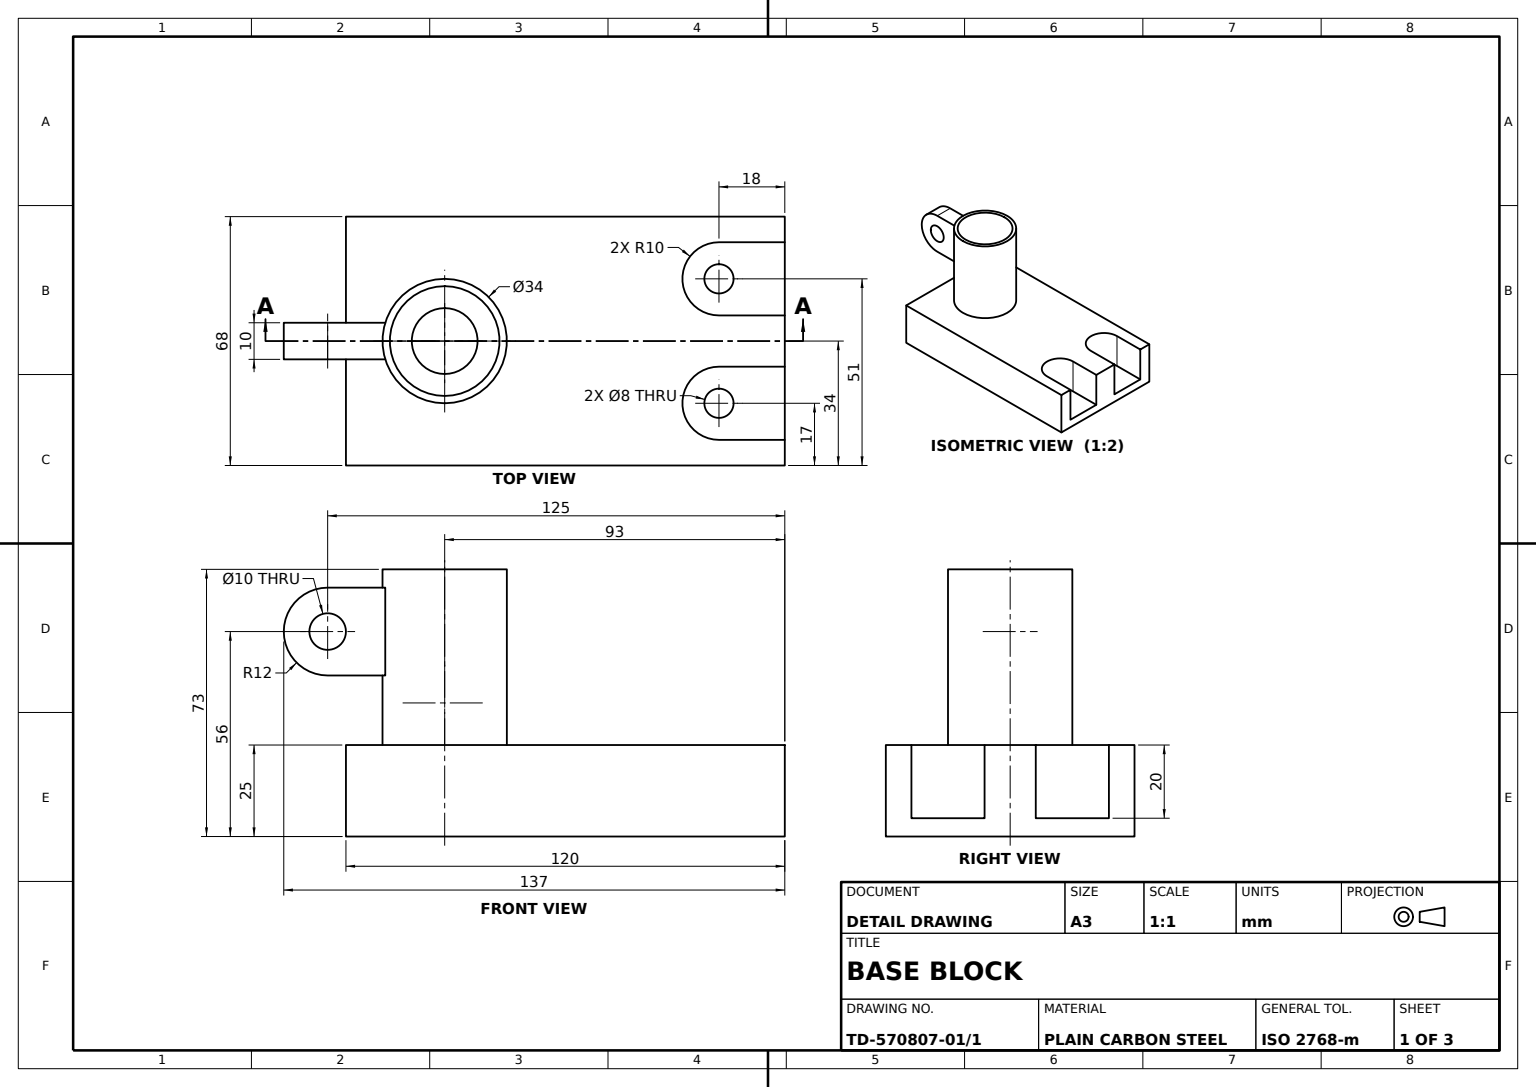
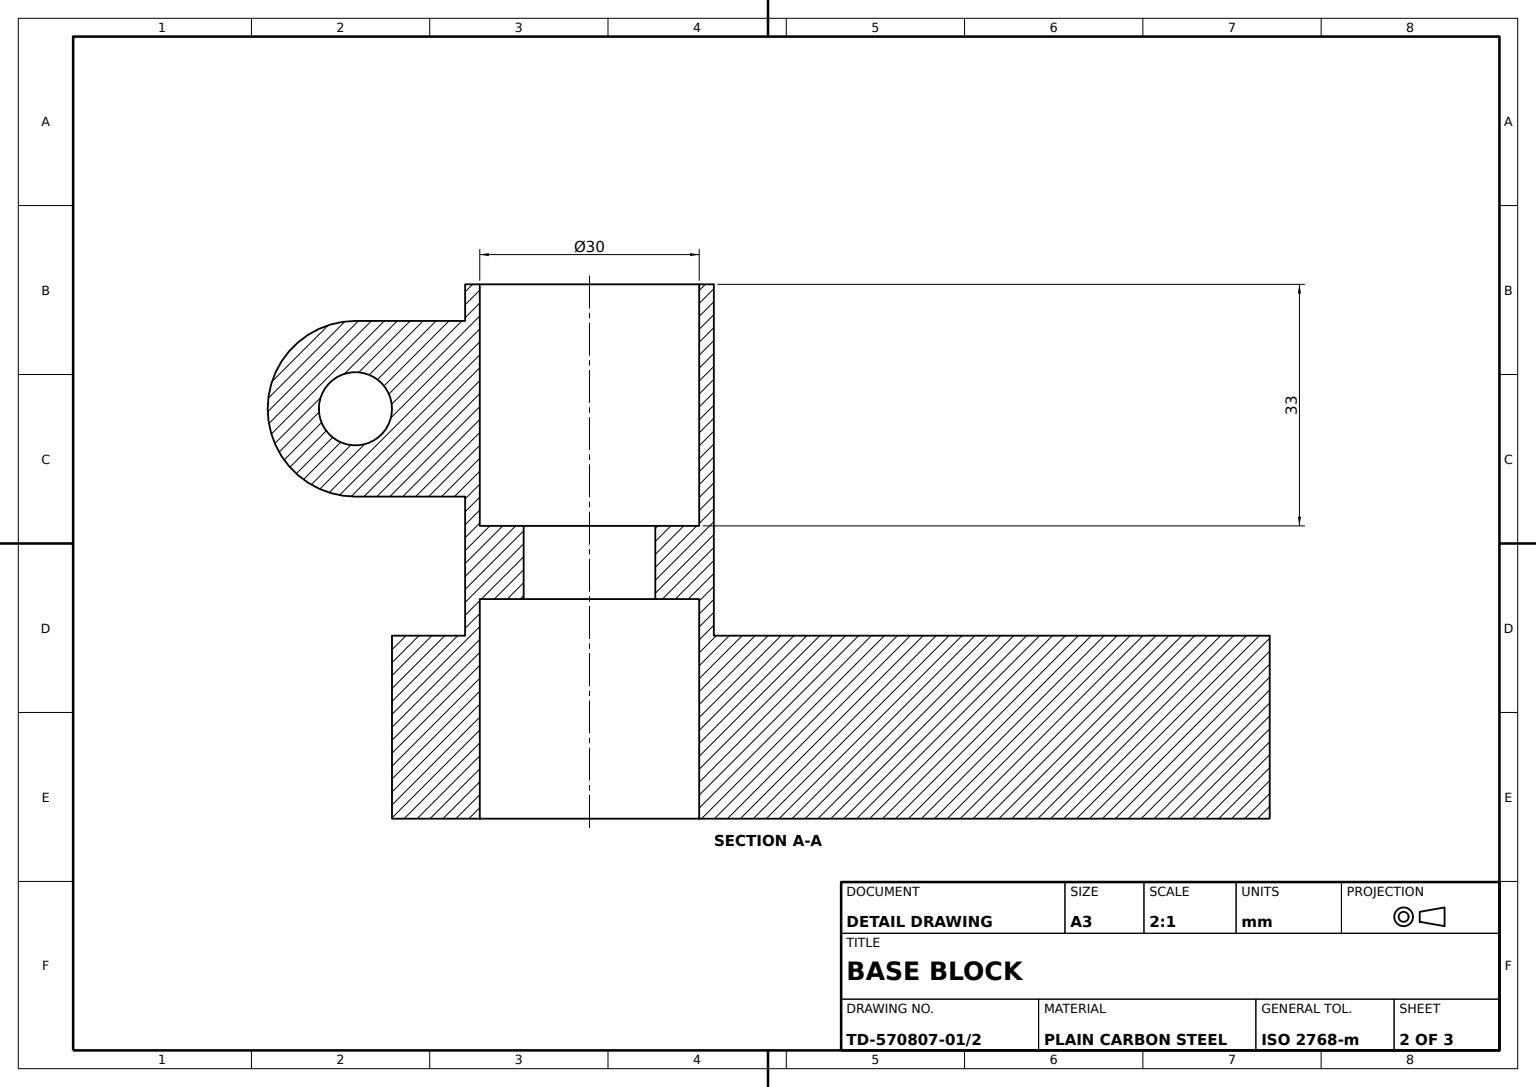
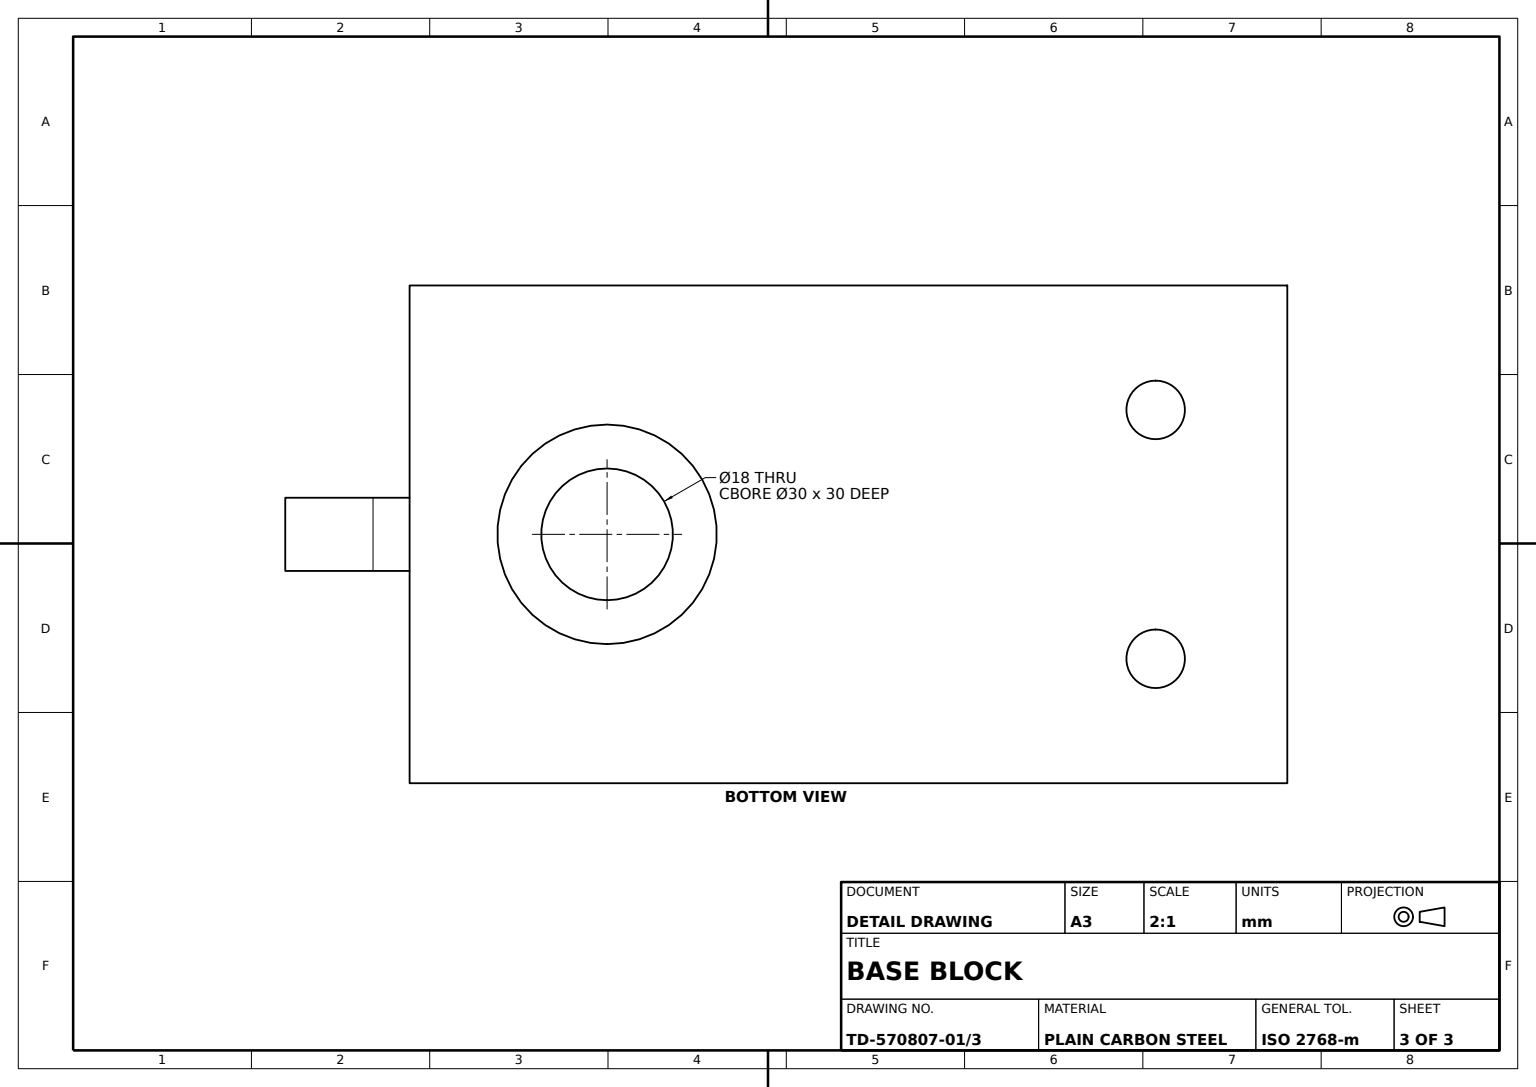
SolidWorks part; units mm, degrees
material "Plain Carbon Steel"
ref_plane "Front Plane" through (0, 0, 0) normal (0, 0, 1) x (1, 0, 0)
ref_plane "Top Plane" through (0, 0, 0) normal (0, 1, 0) x (1, 0, 0)
ref_plane "Right Plane" through (0, 0, 0) normal (1, 0, 0) x (0, 0, -1)
sketch "Base Plate Sketch" plane through (0, 0, 0) normal (0, 1, 0) x (1, 0, 0)
  line L1 (-60, -34) -> (60, -34)
  line L2 (-60, -34) -> (-60, 34)
  line L3 (-60, 34) -> (60, 34)
  line L4 (60, -34) -> (60, 34)
  line L5 (-60, -34) -> (60, 34) construction
  line L6 (-60, 34) -> (60, -34) construction
  point P0 (0, 0)
  dimension "D1" = 120
  dimension "D2" = 68
extrude "Base Plate" add sketch "Base Plate Sketch" along normal blind 25
sketch "Hub Sketch" plane through (0, 25, 0) normal (0, 1, 0) x (1, 0, 0)
  circle A0 centre (-33, 0) radius 17
  dimension "D1" = 34
  dimension "D2" = 93
  dimension "D3" = 34
extrude "Hub Ø34" add sketch "Hub Sketch" along normal blind 48
ref_plane "Lug Plane" through (0, 0, 0) normal (0, 0, 1) x (1, 0, 0)
sketch "Lug Sketch" plane through (0, 0, 0) normal (0, 0, 1) x (1, 0, 0)
  line L0 (-65, 68) -> (-48.8984, 68)
  line L1 (-48.8984, 68) -> (-48.8984, 44)
  line L2 (-48.8984, 44) -> (-65, 44)
  arc A0 (-65, 68) -> (-65, 44) centre (-65, 56) ccw
  dimension "D1" = 24
  dimension "D2" = 56
  dimension "D3" = 125
  dimension "D4" = 16.1016
extrude "Lug" add sketch "Lug Sketch" along normal mid plane 10
sketch "Hub Bore Sketch" plane through (0, 73, 0) normal (0, 1, 0) x (1, 0, 0)
  circle A0 centre (-33, 0) radius 15
  dimension "D1" = 30
extrude "Hub Bore Ø30" cut sketch "Hub Bore Sketch" against normal blind 33
sketch "Through Hole Sketch" plane through (0, 40, 0) normal (0, 1, 0) x (1, 0, 0)
  circle A0 centre (-33, 0) radius 9
  dimension "D1" = 18
extrude "Through Hole Ø18" cut sketch "Through Hole Sketch" against normal blind 10
ref_plane "Bottom Bore Plane" through (0, 30, 0) normal (0, 1, 0) x (1, 0, 0)
sketch "Bottom Bore Sketch" plane through (0, 30, 0) normal (0, 1, 0) x (1, 0, 0)
  circle A0 centre (-33, 0) radius 15
  dimension "D1" = 30
extrude "Bottom Bore Ø30" cut sketch "Bottom Bore Sketch" against normal through all
sketch "Lug Hole Sketch" plane through (0, 0, 5) normal (0, 0, 1) x (1, 0, 0)
  circle A0 centre (-65, 56) radius 5
  dimension "D1" = 10
extrude "Lug Hole Ø10" cut sketch "Lug Hole Sketch" against normal blind 25
sketch "Mounting Slots Sketch" plane through (0, 25, 0) normal (0, 1, 0) x (1, 0, 0)
  line L0 (60, 34) -> (-60, 34) construction
  line L1 (-60, -34) -> (60, -34) construction
  line L2 (60, -34) -> (60, 34) construction
  line L3 (42, 27) -> (60, 27)
  line L4 (60, 27) -> (60, 7)
  line L5 (60, 7) -> (42, 7)
  line L6 (42, -7) -> (60, -7)
  line L7 (60, -7) -> (60, -27)
  line L8 (60, -27) -> (42, -27)
  arc A0 (42, 27) -> (42, 7) centre (42, 17) ccw
  arc A1 (42, -7) -> (42, -27) centre (42, -17) ccw
  dimension "D1" = 20
  dimension "D2" = 20
  dimension "D3" = 34
  dimension "D4" = 17
  dimension "D5" = 17
  dimension "D6" = 18
extrude "Mounting Slots 2x20" cut sketch "Mounting Slots Sketch" against normal blind 20
sketch "Slot Relief Sketch" plane through (0, 5, 0) normal (0, 1, 0) x (1, 0, 0)
  circle A0 centre (42, 17) radius 4
  circle A1 centre (42, -17) radius 4
  dimension "D1" = 8
  dimension "D2" = 8
extrude "Slot Relief Cuts" cut sketch "Slot Relief Sketch" against normal blind 20
